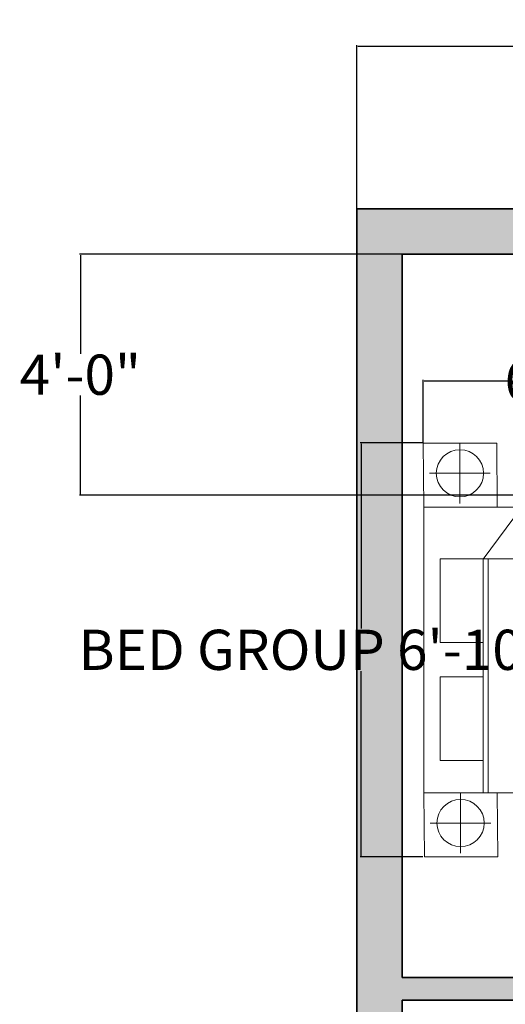
# Model space of a CAD drawing. Units: inches. Extents: x -4737294 to -4736756, y 1716389 to 1717040.
# Tile 19 of 25: x -4737282 to -4737186, y 1716844 to 1717040. Entities that reach past the tile are written whole.
import ezdxf

# ---------------------------------------------------------------- set-up
doc = ezdxf.new("R2010")
doc.units = ezdxf.units.IN
doc.header["$MEASUREMENT"] = 0
for name, color, linetype, lineweight in [('A-ANNO-DIMS', 2, 'Continuous', 18), ('A-WALL-PATT', 244, 'Continuous', 13), ('furniture', 250, 'Continuous', 18), ('walls', 252, 'Continuous', 35)]:
    doc.layers.add(name, color=color, linetype=linetype, lineweight=lineweight)
doc.styles.get("Standard").update_dxf_attribs({"font": 'arial.ttf'})
doc.dimstyles.get("Standard").update_dxf_attribs({"dimtxt": 8, "dimasz": 0.18, "dimexe": 0.18, "dimexo": 0.0625, "dimgap": 0.09, "dimtad": 0, "dimtih": 1, "dimtoh": 1, "dimzin": 0, "dimdsep": 46, "dimlunit": 3, "dimtxsty": 'Standard', "dimcen": 0.09, "dimadec": 0, "dimazin": 0, "dimtfac": 1, "dimtofl": 0, "dimtmove": 0, "dimatfit": 3, "dimfxl": 1, "dimtolj": 1, "dimtzin": 0, "dimarcsym": 0})

# ---------------------------------------------------------------- blocks, each defined once
blk = doc.blocks.new('*D21')
at = {"layer": 'A-ANNO-DIMS', "color": 0, "lineweight": -2, "transparency": 16777216}
for p, q in [((-4737215.14, 1717002.13), (-4737215.14, 1717034.64)), ((-4737214.96, 1717034.46), (-4737042.02, 1717034.46)), ((-4736855.32, 1717034.46), (-4737028.27, 1717034.46)), ((-4736855.14, 1717002.13), (-4736855.14, 1717034.64))]:
    blk.add_line(p, q, dxfattribs=at)
at = {"layer": 'A-ANNO-DIMS', "color": 0, "transparency": 16777216}
for points in [[(-4737214.96, 1717034.49), (-4737214.96, 1717034.43), (-4737215.14, 1717034.46)], [(-4736855.32, 1717034.49), (-4736855.32, 1717034.43), (-4736855.14, 1717034.46)]]:
    blk.add_solid(points, dxfattribs=at)
at = {"layer": 'Defpoints', "color": 0, "transparency": 16777216}
for p in [(-4736855.14, 1717034.46), (-4737215.14, 1717002.06), (-4736855.14, 1717002.06)]:
    blk.add_point(p, dxfattribs=at)
at = {"layer": 'A-ANNO-DIMS', "color": 0, "transparency": 16777216, "insert": (-4737035.14, 1717034.46), "char_height": 8, "attachment_point": 5}
blk.add_mtext("\\A1;30'", dxfattribs=at)
blk = doc.blocks.new('CARPET')
at = {"layer": 'furniture'}
for p, q in [((-51.53, -98.11), (-51.53, -55.12)), ((-51.53, -55.12), (-41.27, -55.12)), ((36, -55.12), (51.55, -55.12)), ((51.55, -55.12), (51.55, -98.11)), ((51.55, -98.11), (-51.53, -98.11))]:
    blk.add_line(p, q, dxfattribs=at)
for points, knots in [([(-53.37, -55.99), (-53.22, -55.8), (-52.9, -55.41), (-52.34, -55.8), (-51.89, -56.08), (-51.65, -55.91), (-51.53, -55.83)], [0, 0, 0, 0, 0.653278, 1.290138, 1.740457, 2.114451, 2.114451, 2.114451, 2.114451]), ([(53.37, -55.99), (53.22, -55.8), (52.9, -55.41), (52.34, -55.8), (51.89, -56.08), (51.65, -55.91), (51.53, -55.83)], [0, 0, 0, 0, 0.653278, 1.290138, 1.740457, 2.114451, 2.114451, 2.114451, 2.114451]), ([(-53.37, -57.26), (-53.22, -57.07), (-52.9, -56.67), (-52.34, -57.07), (-51.89, -57.35), (-51.65, -57.17), (-51.53, -57.1)], [0, 0, 0, 0, 0.653278, 1.290138, 1.740457, 2.114451, 2.114451, 2.114451, 2.114451]), ([(-53.37, -58.59), (-53.22, -58.4), (-52.9, -58.01), (-52.34, -58.4), (-51.89, -58.68), (-51.65, -58.5), (-51.53, -58.43)], [0, 0, 0, 0, 0.653278, 1.290138, 1.740457, 2.114451, 2.114451, 2.114451, 2.114451]), ([(53.37, -57.26), (53.22, -57.07), (52.9, -56.67), (52.34, -57.07), (51.89, -57.35), (51.65, -57.17), (51.53, -57.1)], [0, 0, 0, 0, 0.653278, 1.290138, 1.740457, 2.114451, 2.114451, 2.114451, 2.114451]), ([(53.37, -58.59), (53.22, -58.4), (52.9, -58.01), (52.34, -58.4), (51.89, -58.68), (51.65, -58.5), (51.53, -58.43)], [0, 0, 0, 0, 0.653278, 1.290138, 1.740457, 2.114451, 2.114451, 2.114451, 2.114451]), ([(-53.37, -59.78), (-53.22, -59.58), (-52.9, -59.19), (-52.34, -59.58), (-51.89, -59.86), (-51.65, -59.69), (-51.53, -59.61)], [0, 0, 0, 0, 0.653278, 1.290138, 1.740457, 2.114451, 2.114451, 2.114451, 2.114451]), ([(-53.37, -61.22), (-53.22, -61.02), (-52.9, -60.63), (-52.34, -61.02), (-51.89, -61.3), (-51.65, -61.13), (-51.53, -61.05)], [0, 0, 0, 0, 0.653278, 1.290138, 1.740457, 2.114451, 2.114451, 2.114451, 2.114451]), ([(53.37, -59.78), (53.22, -59.58), (52.9, -59.19), (52.34, -59.58), (51.89, -59.86), (51.65, -59.69), (51.53, -59.61)], [0, 0, 0, 0, 0.653278, 1.290138, 1.740457, 2.114451, 2.114451, 2.114451, 2.114451]), ([(53.37, -61.22), (53.22, -61.02), (52.9, -60.63), (52.34, -61.02), (51.89, -61.3), (51.65, -61.13), (51.53, -61.05)], [0, 0, 0, 0, 0.653278, 1.290138, 1.740457, 2.114451, 2.114451, 2.114451, 2.114451]), ([(-53.37, -62.44), (-53.22, -62.25), (-52.9, -61.86), (-52.34, -62.25), (-51.89, -62.53), (-51.65, -62.36), (-51.53, -62.28)], [0, 0, 0, 0, 0.653278, 1.290138, 1.740457, 2.114451, 2.114451, 2.114451, 2.114451]), ([(-53.37, -63.63), (-53.22, -63.43), (-52.9, -63.04), (-52.34, -63.43), (-51.89, -63.72), (-51.65, -63.54), (-51.53, -63.46)], [0, 0, 0, 0, 0.653278, 1.290138, 1.740457, 2.114451, 2.114451, 2.114451, 2.114451]), ([(53.37, -62.44), (53.22, -62.25), (52.9, -61.86), (52.34, -62.25), (51.89, -62.53), (51.65, -62.36), (51.53, -62.28)], [0, 0, 0, 0, 0.653278, 1.290138, 1.740457, 2.114451, 2.114451, 2.114451, 2.114451]), ([(53.37, -63.63), (53.22, -63.43), (52.9, -63.04), (52.34, -63.43), (51.89, -63.72), (51.65, -63.54), (51.53, -63.46)], [0, 0, 0, 0, 0.653278, 1.290138, 1.740457, 2.114451, 2.114451, 2.114451, 2.114451]), ([(-53.37, -65.07), (-53.22, -64.87), (-52.9, -64.48), (-52.34, -64.87), (-51.89, -65.15), (-51.65, -64.98), (-51.53, -64.9)], [0, 0, 0, 0, 0.653278, 1.290138, 1.740457, 2.114451, 2.114451, 2.114451, 2.114451]), ([(-53.37, -66.76), (-53.22, -66.56), (-52.9, -66.17), (-52.34, -66.56), (-51.89, -66.84), (-51.65, -66.67), (-51.53, -66.59)], [0, 0, 0, 0, 0.653278, 1.290138, 1.740457, 2.114451, 2.114451, 2.114451, 2.114451]), ([(53.37, -65.07), (53.22, -64.87), (52.9, -64.48), (52.34, -64.87), (51.89, -65.15), (51.65, -64.98), (51.53, -64.9)], [0, 0, 0, 0, 0.653278, 1.290138, 1.740457, 2.114451, 2.114451, 2.114451, 2.114451]), ([(53.37, -66.76), (53.22, -66.56), (52.9, -66.17), (52.34, -66.56), (51.89, -66.84), (51.65, -66.67), (51.53, -66.59)], [0, 0, 0, 0, 0.653278, 1.290138, 1.740457, 2.114451, 2.114451, 2.114451, 2.114451]), ([(-53.37, -68.2), (-53.22, -68), (-52.9, -67.61), (-52.34, -68), (-51.89, -68.28), (-51.65, -68.11), (-51.53, -68.03)], [0, 0, 0, 0, 0.653278, 1.290138, 1.740457, 2.114451, 2.114451, 2.114451, 2.114451]), ([(-53.37, -69.53), (-53.22, -69.33), (-52.9, -68.94), (-52.34, -69.33), (-51.89, -69.61), (-51.65, -69.44), (-51.53, -69.36)], [0, 0, 0, 0, 0.653278, 1.290138, 1.740457, 2.114451, 2.114451, 2.114451, 2.114451]), ([(53.37, -68.2), (53.22, -68), (52.9, -67.61), (52.34, -68), (51.89, -68.28), (51.65, -68.11), (51.53, -68.03)], [0, 0, 0, 0, 0.653278, 1.290138, 1.740457, 2.114451, 2.114451, 2.114451, 2.114451]), ([(53.37, -69.53), (53.22, -69.33), (52.9, -68.94), (52.34, -69.33), (51.89, -69.61), (51.65, -69.44), (51.53, -69.36)], [0, 0, 0, 0, 0.653278, 1.290138, 1.740457, 2.114451, 2.114451, 2.114451, 2.114451]), ([(-53.37, -70.79), (-53.22, -70.6), (-52.9, -70.21), (-52.34, -70.6), (-51.89, -70.88), (-51.65, -70.7), (-51.53, -70.63)], [0, 0, 0, 0, 0.653278, 1.290138, 1.740457, 2.114451, 2.114451, 2.114451, 2.114451]), ([(-53.37, -72.12), (-53.22, -71.93), (-52.9, -71.54), (-52.34, -71.93), (-51.89, -72.21), (-51.65, -72.04), (-51.53, -71.96)], [0, 0, 0, 0, 0.653278, 1.290138, 1.740457, 2.114451, 2.114451, 2.114451, 2.114451]), ([(53.37, -70.79), (53.22, -70.6), (52.9, -70.21), (52.34, -70.6), (51.89, -70.88), (51.65, -70.7), (51.53, -70.63)], [0, 0, 0, 0, 0.653278, 1.290138, 1.740457, 2.114451, 2.114451, 2.114451, 2.114451]), ([(53.37, -72.12), (53.22, -71.93), (52.9, -71.54), (52.34, -71.93), (51.89, -72.21), (51.65, -72.04), (51.53, -71.96)], [0, 0, 0, 0, 0.653278, 1.290138, 1.740457, 2.114451, 2.114451, 2.114451, 2.114451]), ([(-53.37, -73.31), (-53.22, -73.11), (-52.9, -72.72), (-52.34, -73.11), (-51.89, -73.4), (-51.65, -73.22), (-51.53, -73.14)], [0, 0, 0, 0, 0.653278, 1.290138, 1.740457, 2.114451, 2.114451, 2.114451, 2.114451]), ([(-53.37, -74.75), (-53.22, -74.55), (-52.9, -74.16), (-52.34, -74.55), (-51.89, -74.83), (-51.65, -74.66), (-51.53, -74.58)], [0, 0, 0, 0, 0.653278, 1.290138, 1.740457, 2.114451, 2.114451, 2.114451, 2.114451]), ([(53.37, -73.31), (53.22, -73.11), (52.9, -72.72), (52.34, -73.11), (51.89, -73.4), (51.65, -73.22), (51.53, -73.14)], [0, 0, 0, 0, 0.653278, 1.290138, 1.740457, 2.114451, 2.114451, 2.114451, 2.114451]), ([(53.37, -74.75), (53.22, -74.55), (52.9, -74.16), (52.34, -74.55), (51.89, -74.83), (51.65, -74.66), (51.53, -74.58)], [0, 0, 0, 0, 0.653278, 1.290138, 1.740457, 2.114451, 2.114451, 2.114451, 2.114451]), ([(-53.37, -75.98), (-53.22, -75.78), (-52.9, -75.39), (-52.34, -75.78), (-51.89, -76.06), (-51.65, -75.89), (-51.53, -75.81)], [0, 0, 0, 0, 0.653278, 1.290138, 1.740457, 2.114451, 2.114451, 2.114451, 2.114451]), ([(-53.37, -77.16), (-53.22, -76.96), (-52.9, -76.57), (-52.34, -76.96), (-51.89, -77.25), (-51.65, -77.07), (-51.53, -76.99)], [0, 0, 0, 0, 0.653278, 1.290138, 1.740457, 2.114451, 2.114451, 2.114451, 2.114451]), ([(53.37, -75.98), (53.22, -75.78), (52.9, -75.39), (52.34, -75.78), (51.89, -76.06), (51.65, -75.89), (51.53, -75.81)], [0, 0, 0, 0, 0.653278, 1.290138, 1.740457, 2.114451, 2.114451, 2.114451, 2.114451]), ([(53.37, -77.16), (53.22, -76.96), (52.9, -76.57), (52.34, -76.96), (51.89, -77.25), (51.65, -77.07), (51.53, -76.99)], [0, 0, 0, 0, 0.653278, 1.290138, 1.740457, 2.114451, 2.114451, 2.114451, 2.114451]), ([(-53.37, -78.6), (-53.22, -78.4), (-52.9, -78.01), (-52.34, -78.4), (-51.89, -78.68), (-51.65, -78.51), (-51.53, -78.43)], [0, 0, 0, 0, 0.653278, 1.290138, 1.740457, 2.114451, 2.114451, 2.114451, 2.114451]), ([(-53.37, -80.29), (-53.22, -80.09), (-52.9, -79.7), (-52.34, -80.09), (-51.89, -80.37), (-51.65, -80.2), (-51.53, -80.12)], [0, 0, 0, 0, 0.653278, 1.290138, 1.740457, 2.114451, 2.114451, 2.114451, 2.114451]), ([(53.37, -78.6), (53.22, -78.4), (52.9, -78.01), (52.34, -78.4), (51.89, -78.68), (51.65, -78.51), (51.53, -78.43)], [0, 0, 0, 0, 0.653278, 1.290138, 1.740457, 2.114451, 2.114451, 2.114451, 2.114451]), ([(53.37, -80.29), (53.22, -80.09), (52.9, -79.7), (52.34, -80.09), (51.89, -80.37), (51.65, -80.2), (51.53, -80.12)], [0, 0, 0, 0, 0.653278, 1.290138, 1.740457, 2.114451, 2.114451, 2.114451, 2.114451]), ([(-53.37, -81.73), (-53.22, -81.53), (-52.9, -81.14), (-52.34, -81.53), (-51.89, -81.81), (-51.65, -81.64), (-51.53, -81.56)], [0, 0, 0, 0, 0.653278, 1.290138, 1.740457, 2.114451, 2.114451, 2.114451, 2.114451]), ([(53.37, -81.73), (53.22, -81.53), (52.9, -81.14), (52.34, -81.53), (51.89, -81.81), (51.65, -81.64), (51.53, -81.56)], [0, 0, 0, 0, 0.653278, 1.290138, 1.740457, 2.114451, 2.114451, 2.114451, 2.114451]), ([(-53.37, -83.06), (-53.22, -82.86), (-52.9, -82.47), (-52.34, -82.86), (-51.89, -83.14), (-51.65, -82.97), (-51.53, -82.89)], [0, 0, 0, 0, 0.653278, 1.290138, 1.740457, 2.114451, 2.114451, 2.114451, 2.114451]), ([(-53.37, -84.18), (-53.22, -83.99), (-52.9, -83.6), (-52.34, -83.99), (-51.89, -84.27), (-51.65, -84.09), (-51.53, -84.02)], [0, 0, 0, 0, 0.653278, 1.290138, 1.740457, 2.114451, 2.114451, 2.114451, 2.114451]), ([(-53.37, -85.51), (-53.22, -85.32), (-52.9, -84.93), (-52.34, -85.32), (-51.89, -85.6), (-51.65, -85.42), (-51.53, -85.35)], [0, 0, 0, 0, 0.653278, 1.290138, 1.740457, 2.114451, 2.114451, 2.114451, 2.114451]), ([(53.37, -83.06), (53.22, -82.86), (52.9, -82.47), (52.34, -82.86), (51.89, -83.14), (51.65, -82.97), (51.53, -82.89)], [0, 0, 0, 0, 0.653278, 1.290138, 1.740457, 2.114451, 2.114451, 2.114451, 2.114451]), ([(53.37, -84.18), (53.22, -83.99), (52.9, -83.6), (52.34, -83.99), (51.89, -84.27), (51.65, -84.09), (51.53, -84.02)], [0, 0, 0, 0, 0.653278, 1.290138, 1.740457, 2.114451, 2.114451, 2.114451, 2.114451]), ([(53.37, -85.51), (53.22, -85.32), (52.9, -84.93), (52.34, -85.32), (51.89, -85.6), (51.65, -85.42), (51.53, -85.35)], [0, 0, 0, 0, 0.653278, 1.290138, 1.740457, 2.114451, 2.114451, 2.114451, 2.114451]), ([(-53.37, -86.7), (-53.22, -86.5), (-52.9, -86.11), (-52.34, -86.5), (-51.89, -86.78), (-51.65, -86.61), (-51.53, -86.53)], [0, 0, 0, 0, 0.653278, 1.290138, 1.740457, 2.114451, 2.114451, 2.114451, 2.114451]), ([(-53.37, -88.14), (-53.22, -87.94), (-52.9, -87.55), (-52.34, -87.94), (-51.89, -88.22), (-51.65, -88.05), (-51.53, -87.97)], [0, 0, 0, 0, 0.653278, 1.290138, 1.740457, 2.114451, 2.114451, 2.114451, 2.114451]), ([(53.37, -86.7), (53.22, -86.5), (52.9, -86.11), (52.34, -86.5), (51.89, -86.78), (51.65, -86.61), (51.53, -86.53)], [0, 0, 0, 0, 0.653278, 1.290138, 1.740457, 2.114451, 2.114451, 2.114451, 2.114451]), ([(53.37, -88.14), (53.22, -87.94), (52.9, -87.55), (52.34, -87.94), (51.89, -88.22), (51.65, -88.05), (51.53, -87.97)], [0, 0, 0, 0, 0.653278, 1.290138, 1.740457, 2.114451, 2.114451, 2.114451, 2.114451]), ([(-53.37, -89.36), (-53.22, -89.17), (-52.9, -88.78), (-52.34, -89.17), (-51.89, -89.45), (-51.65, -89.28), (-51.53, -89.2)], [0, 0, 0, 0, 0.653278, 1.290138, 1.740457, 2.114451, 2.114451, 2.114451, 2.114451]), ([(-53.37, -90.55), (-53.22, -90.35), (-52.9, -89.96), (-52.34, -90.35), (-51.89, -90.64), (-51.65, -90.46), (-51.53, -90.38)], [0, 0, 0, 0, 0.653278, 1.290138, 1.740457, 2.114451, 2.114451, 2.114451, 2.114451]), ([(53.37, -89.36), (53.22, -89.17), (52.9, -88.78), (52.34, -89.17), (51.89, -89.45), (51.65, -89.28), (51.53, -89.2)], [0, 0, 0, 0, 0.653278, 1.290138, 1.740457, 2.114451, 2.114451, 2.114451, 2.114451]), ([(53.37, -90.55), (53.22, -90.35), (52.9, -89.96), (52.34, -90.35), (51.9, -90.63), (51.66, -90.47), (51.55, -90.4)], [0, 0, 0, 0, 0.653278, 1.290138, 1.740457, 2.0926, 2.0926, 2.0926, 2.0926]), ([(-53.37, -91.99), (-53.22, -91.79), (-52.9, -91.4), (-52.34, -91.79), (-51.89, -92.07), (-51.65, -91.9), (-51.53, -91.82)], [0, 0, 0, 0, 0.653278, 1.290138, 1.740457, 2.114451, 2.114451, 2.114451, 2.114451]), ([(-53.37, -92.69), (-53.22, -92.48), (-52.9, -92.08), (-52.35, -92.49), (-51.89, -92.77), (-51.65, -92.6), (-51.53, -92.52)], [0, 0, 0, 0, 0.663904, 1.307406, 1.757725, 2.131719, 2.131719, 2.131719, 2.131719]), ([(-53.37, -93.61), (-53.22, -93.42), (-52.9, -93.03), (-52.34, -93.42), (-51.89, -93.7), (-51.65, -93.52), (-51.53, -93.45)], [0, 0, 0, 0, 0.653278, 1.290138, 1.740457, 2.114451, 2.114451, 2.114451, 2.114451]), ([(53.37, -91.99), (53.22, -91.79), (52.9, -91.4), (52.34, -91.79), (51.9, -92.07), (51.66, -91.91), (51.55, -91.83)], [0, 0, 0, 0, 0.653278, 1.290138, 1.740457, 2.0926, 2.0926, 2.0926, 2.0926]), ([(53.37, -92.69), (53.22, -92.49), (52.9, -92.09), (52.34, -92.49), (51.9, -92.77), (51.66, -92.61), (51.55, -92.53)], [0, 0, 0, 0, 0.656792, 1.295826, 1.746145, 2.098292, 2.098292, 2.098292, 2.098292]), ([(53.37, -93.66), (53.22, -93.46), (52.9, -93.07), (52.34, -93.46), (51.9, -93.74), (51.66, -93.58), (51.55, -93.5)], [0, 0, 0, 0, 0.653278, 1.290138, 1.740457, 2.0926, 2.0926, 2.0926, 2.0926]), ([(-53.37, -94.55), (-53.22, -94.35), (-52.9, -93.96), (-52.34, -94.35), (-51.89, -94.63), (-51.65, -94.46), (-51.53, -94.38)], [0, 0, 0, 0, 0.653278, 1.290138, 1.740457, 2.114451, 2.114451, 2.114451, 2.114451]), ([(-53.37, -95.05), (-53.22, -94.85), (-52.9, -94.46), (-52.34, -94.85), (-51.89, -95.14), (-51.65, -94.96), (-51.53, -94.88)], [0, 0, 0, 0, 0.653278, 1.290138, 1.740457, 2.114451, 2.114451, 2.114451, 2.114451]), ([(-53.37, -95.73), (-53.22, -95.54), (-52.9, -95.15), (-52.34, -95.54), (-51.89, -95.82), (-51.65, -95.65), (-51.53, -95.57)], [0, 0, 0, 0, 0.653278, 1.290138, 1.740457, 2.114451, 2.114451, 2.114451, 2.114451]), ([(53.37, -95.78), (53.22, -95.58), (52.9, -95.19), (52.34, -95.58), (51.89, -95.86), (51.65, -95.69), (51.53, -95.61)], [0, 0, 0, 0, 0.653278, 1.290138, 1.740457, 2.114451, 2.114451, 2.114451, 2.114451]), ([(53.37, -94.59), (53.22, -94.4), (52.9, -94.01), (52.34, -94.4), (51.9, -94.68), (51.66, -94.51), (51.55, -94.44)], [0, 0, 0, 0, 0.653278, 1.290138, 1.740457, 2.0926, 2.0926, 2.0926, 2.0926]), ([(53.37, -95.1), (53.22, -94.9), (52.9, -94.51), (52.34, -94.9), (51.9, -95.18), (51.66, -95.02), (51.55, -94.94)], [0, 0, 0, 0, 0.653278, 1.290138, 1.740457, 2.0926, 2.0926, 2.0926, 2.0926]), ([(-53.37, -96.38), (-53.22, -96.18), (-52.9, -95.79), (-52.34, -96.18), (-51.89, -96.47), (-51.65, -96.29), (-51.53, -96.21)], [0, 0, 0, 0, 0.653278, 1.290138, 1.740457, 2.114451, 2.114451, 2.114451, 2.114451]), ([(-53.37, -97.17), (-53.22, -96.98), (-52.9, -96.59), (-52.34, -96.98), (-51.89, -97.26), (-51.65, -97.08), (-51.53, -97.01)], [0, 0, 0, 0, 0.653278, 1.290138, 1.740457, 2.114451, 2.114451, 2.114451, 2.114451]), ([(-53.37, -97.99), (-53.22, -97.79), (-52.9, -97.4), (-52.34, -97.79), (-51.89, -98.08), (-51.65, -97.9), (-51.53, -97.82)], [0, 0, 0, 0, 0.653278, 1.290138, 1.740457, 2.114451, 2.114451, 2.114451, 2.114451]), ([(53.37, -96.43), (53.22, -96.23), (52.9, -95.84), (52.34, -96.23), (51.89, -96.51), (51.65, -96.34), (51.53, -96.26)], [0, 0, 0, 0, 0.653278, 1.290138, 1.740457, 2.114451, 2.114451, 2.114451, 2.114451]), ([(53.37, -97.22), (53.22, -97.02), (52.9, -96.63), (52.34, -97.02), (51.89, -97.3), (51.65, -97.13), (51.53, -97.05)], [0, 0, 0, 0, 0.653278, 1.290138, 1.740457, 2.114451, 2.114451, 2.114451, 2.114451]), ([(53.37, -97.99), (53.22, -97.79), (52.9, -97.4), (52.34, -97.79), (51.89, -98.08), (51.65, -97.9), (51.53, -97.82)], [0, 0, 0, 0, 0.653278, 1.290138, 1.740457, 2.114451, 2.114451, 2.114451, 2.114451])]:
    blk.add_open_spline(points, degree=3, knots=knots, dxfattribs=at)
blk = doc.blocks.new('A$C58D270C6')
at = {"layer": 'furniture'}
for p, q in [((9.09, 124.13), (9.09, 108.87)), ((1.46, 116.5), (16.73, 116.5)), ((14.97, 94.84), (24.62, 107.92)), ((24.62, 94.93), (24.62, 107.92)), ((42.08, 108), (42.08, 36)), ((14.97, 94.93), (24.62, 94.93)), ((14.97, 94.84), (14.97, 36)), ((16.22, 94.93), (16.22, 36)), ((9.25, 36), (9.25, 20.74)), ((1.62, 28.37), (16.88, 28.37))]:
    blk.add_line(p, q, dxfattribs=at)
for points in [[(18.5, 108), (18.34, 124.13), (-0.16, 124.13), (0, 108)], [(0, 108), (77.91, 108), (77.91, 36), (0, 36)], [(4.09, 94.93), (14.97, 94.93), (14.97, 73.83), (4.09, 73.83)], [(4.09, 65.23), (14.97, 65.23), (14.97, 44.13), (4.09, 44.13)], [(18.65, 19.87), (18.5, 36), (0, 36), (0.16, 19.87)]]:
    blk.add_lwpolyline(points, close=True, dxfattribs=at)
for centre in [(9.09, 116.5), (9.25, 28.37)]:
    blk.add_circle(centre, 5.95, dxfattribs=at)
at = {"layer": 'furniture', "xscale": 0.9312884925094044, "yscale": 0.9312884925094044, "zscale": 0.9312884925094044, "rotation": 90}
blk.add_blockref('CARPET', (3.79, 74.47), dxfattribs=at)
blk = doc.blocks.new('*D31')
at = {"layer": 'A-ANNO-DIMS', "color": 0, "lineweight": -2, "transparency": 16777216}
for p, q in [((-4737202.03, 1716955.51), (-4737214.51, 1716955.51)), ((-4737214.33, 1716955.33), (-4737214.33, 1716918.54)), ((-4737214.33, 1716873.3), (-4737214.33, 1716910.08)), ((-4737202.03, 1716873.12), (-4737214.51, 1716873.12))]:
    blk.add_line(p, q, dxfattribs=at)
at = {"layer": 'A-ANNO-DIMS', "color": 0, "transparency": 16777216}
for points in [[(-4737214.36, 1716955.33), (-4737214.3, 1716955.33), (-4737214.33, 1716955.51)], [(-4737214.36, 1716873.3), (-4737214.3, 1716873.3), (-4737214.33, 1716873.12)]]:
    blk.add_solid(points, dxfattribs=at)
at = {"layer": 'Defpoints', "color": 0, "transparency": 16777216}
for p in [(-4737214.33, 1716955.51), (-4737201.97, 1716955.51), (-4737201.97, 1716873.12)]:
    blk.add_point(p, dxfattribs=at)
at = {"layer": 'A-ANNO-DIMS', "color": 0, "transparency": 16777216, "insert": (-4737214.33, 1716914.31), "char_height": 8, "attachment_point": 5}
blk.add_mtext('\\A1;BED GROUP 6\'-10 1/2"', dxfattribs=at)
blk = doc.blocks.new('*D32')
at = {"layer": 'A-ANNO-DIMS', "color": 0, "lineweight": -2, "transparency": 16777216}
for p, q in [((-4737201.97, 1716955.57), (-4737201.97, 1716968.04)), ((-4737201.79, 1716967.86), (-4737184.4, 1716967.86)), ((-4737126.87, 1716967.86), (-4737144.27, 1716967.86)), ((-4737126.69, 1716955.57), (-4737126.69, 1716968.04))]:
    blk.add_line(p, q, dxfattribs=at)
at = {"layer": 'A-ANNO-DIMS', "color": 0, "transparency": 16777216}
for points in [[(-4737201.79, 1716967.89), (-4737201.79, 1716967.83), (-4737201.97, 1716967.86)], [(-4737126.87, 1716967.89), (-4737126.87, 1716967.83), (-4737126.69, 1716967.86)]]:
    blk.add_solid(points, dxfattribs=at)
at = {"layer": 'Defpoints', "color": 0, "transparency": 16777216}
for p in [(-4737126.69, 1716967.86), (-4737201.97, 1716955.51), (-4737126.69, 1716955.51)]:
    blk.add_point(p, dxfattribs=at)
at = {"layer": 'A-ANNO-DIMS', "color": 0, "transparency": 16777216, "insert": (-4737164.33, 1716967.86), "char_height": 8, "attachment_point": 5}
blk.add_mtext('\\A1;6\'-3 1/2"', dxfattribs=at)
blk = doc.blocks.new('*D70')
at = {"layer": 'A-ANNO-DIMS', "color": 0, "lineweight": -2, "transparency": 16777216}
for p, q in [((-4737056.78, 1716993.06), (-4737270.32, 1716993.06)), ((-4737270.14, 1716992.88), (-4737270.14, 1716973.24)), ((-4737270.14, 1716945.24), (-4737270.14, 1716964.89)), ((-4737056.78, 1716945.06), (-4737270.32, 1716945.06))]:
    blk.add_line(p, q, dxfattribs=at)
at = {"layer": 'A-ANNO-DIMS', "color": 0, "transparency": 16777216}
for points in [[(-4737270.17, 1716992.88), (-4737270.11, 1716992.88), (-4737270.14, 1716993.06)], [(-4737270.17, 1716945.24), (-4737270.11, 1716945.24), (-4737270.14, 1716945.06)]]:
    blk.add_solid(points, dxfattribs=at)
at = {"layer": 'Defpoints', "color": 0, "transparency": 16777216}
for p in [(-4737056.72, 1716993.06), (-4737270.14, 1716945.06), (-4737056.72, 1716945.06)]:
    blk.add_point(p, dxfattribs=at)
at = {"layer": 'A-ANNO-DIMS', "color": 0, "transparency": 16777216, "insert": (-4737270.14, 1716969.06), "char_height": 8, "attachment_point": 5}
blk.add_mtext('\\A1;4\'-0"', dxfattribs=at)

msp = doc.modelspace()

# ---------------------------------------------------------------- hatches: boundary and pattern name
at = {"layer": 'A-WALL-PATT'}
h = msp.add_hatch(color=256, dxfattribs=at)
h.dxf.hatch_style = 1
h.paths.add_polyline_path([(-4737206.144, 1716844.565), (-4737110.144, 1716844.565), (-4737110.144, 1716823.907), (-4737105.644, 1716823.907), (-4737105.644, 1716844.565), (-4737098.44, 1716844.565), (-4737098.44, 1716849.065), (-4737206.144, 1716849.065), (-4737206.144, 1716993.065), (-4736864.144, 1716993.065), (-4736864.144, 1716849.065), (-4736963.275, 1716849.065), (-4736994.446, 1716849.065), (-4736997.144, 1716849.065), (-4736997.144, 1716844.565), (-4736864.144, 1716844.565), (-4736864.144, 1716668.565), (-4736934.391, 1716668.565), (-4736934.391, 1716664.065), (-4736864.144, 1716664.065), (-4736864.144, 1716462.065), (-4736855.144, 1716462.065), (-4736855.144, 1717002.065), (-4737215.144, 1717002.065), (-4737215.144, 1716462.065), (-4737206.144, 1716462.065), (-4737206.144, 1716659.065), (-4737062.144, 1716659.065), (-4737062.144, 1716647.493), (-4737057.644, 1716647.493), (-4737057.644, 1716796.565), (-4737071.812, 1716796.565), (-4737071.812, 1716792.065), (-4737070.805, 1716792.065), (-4737062.144, 1716792.065), (-4737062.144, 1716668.065), (-4737206.144, 1716668.065), (-4737206.144, 1716792.065), (-4737093.784, 1716792.065), (-4737093.784, 1716796.565), (-4737206.144, 1716796.565)])

# ---------------------------------------------------------------- linework, layer by layer
at = {"layer": 'walls'}
for p, q in [((-4737215.144, 1717002.065), (-4736855.144, 1717002.065)), ((-4737215.144, 1716462.065), (-4737215.144, 1717002.065)), ((-4737215.144, 1717002.065), (-4737215.144, 1717002.065)), ((-4737206.144, 1716993.065), (-4736864.144, 1716993.065)), ((-4737206.144, 1716849.065), (-4737206.144, 1716993.065)), ((-4737206.144, 1716849.065), (-4737097.919, 1716849.065)), ((-4737206.144, 1716844.565), (-4737110.144, 1716844.565)), ((-4737206.144, 1716844.565), (-4737110.144, 1716844.565)), ((-4737206.144, 1716796.565), (-4737206.144, 1716844.565))]:
    msp.add_line(p, q, dxfattribs=at)

# ---------------------------------------------------------------- block references
at = {"layer": 'furniture', "xscale": 0.7897983012973059, "yscale": 0.7897983012973059, "zscale": 0.7897983012973059}
msp.add_blockref('A$C58D270C6', (-4737201.848, 1716857.428), dxfattribs=at)

# ---------------------------------------------------------------- dimensions: what is measured, and where the dimension line sits
at = {"layer": 'A-ANNO-DIMS'}
for base, p1, p2, override, picture, middle in [((-4736855.144, 1717034.458), (-4737215.144, 1717002.065), (-4736855.144, 1717002.065), {"dimclrd": 0, "dimclre": 0, "dimclrt": 0}, '*D21', (-4737035.144, 1717034.458)), ((-4737126.692, 1716967.863), (-4737201.971, 1716955.505), (-4737126.692, 1716955.505), {"dimdec": 1, "dimlfac": 1, "dimrnd": 0, "dimzin": 1, "dimdsep": 46, "dimlunit": 4, "dimfrac": 2}, '*D32', (-4737164.331, 1716967.863))]:
    dim = msp.add_linear_dim(base=base, p1=p1, p2=p2, dimstyle='Standard', override=override, dxfattribs=at)
    dim.commit()
    dim.dimension.update_dxf_attribs({"geometry": picture, "text_midpoint": middle})
dim = msp.add_linear_dim(base=(-4737270.144, 1716945.065), p1=(-4737056.719, 1716993.065), p2=(-4737056.719, 1716945.065), angle=90, dimstyle='Standard', override={"dimdec": 1, "dimlfac": 1, "dimrnd": 0, "dimzin": 1, "dimdsep": 46, "dimlunit": 4, "dimfrac": 2}, dxfattribs=at)
dim.commit()
dim.dimension.update_dxf_attribs({"geometry": '*D70', "text_midpoint": (-4737270.144, 1716969.065)})
dim = msp.add_linear_dim(base=(-4737214.329, 1716955.505), p1=(-4737201.971, 1716873.12), p2=(-4737201.971, 1716955.505), angle=90, text='BED GROUP <>', dimstyle='Standard', override={"dimdec": 1, "dimlfac": 1, "dimrnd": 0, "dimzin": 1, "dimdsep": 46, "dimlunit": 4, "dimfrac": 2}, dxfattribs=at)
dim.commit()
dim.dimension.update_dxf_attribs({"geometry": '*D31', "text_midpoint": (-4737214.329, 1716914.313)})

doc.saveas('drawing.dxf')
